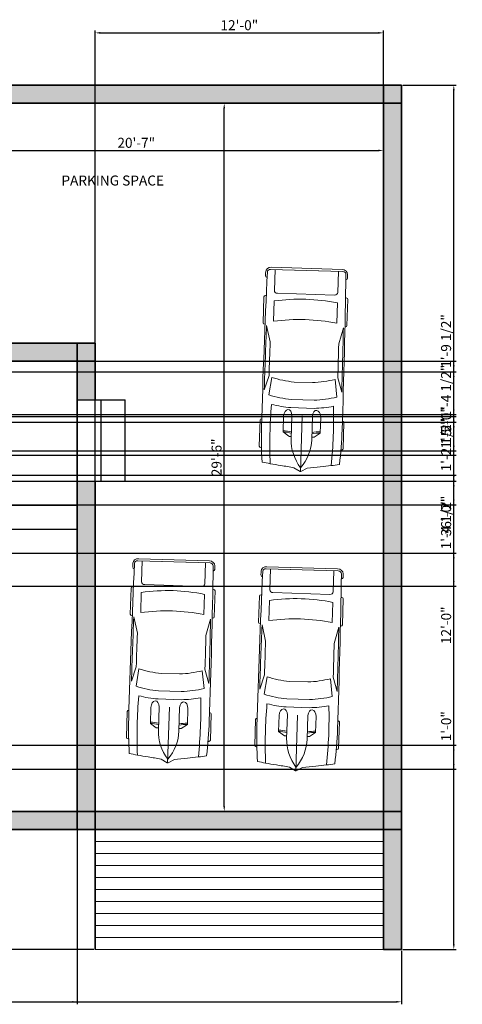
# Model space of a CAD drawing. Units: millimetres. Extents: x 2803 to 3393, y 965 to 1464.
# Tile 6 of 6: x 3172 to 3393, y 968 to 1460. Entities that reach past the tile are written whole.
import ezdxf

# ---------------------------------------------------------------- set-up
doc = ezdxf.new("R2010")
doc.units = ezdxf.units.MM
for name, color, linetype, lineweight in [('A-ANNO-DIMS', 150, 'Continuous', 18), ('A-AREA-IDEN', 200, 'Continuous', 25), ('A-SITE-PVMT', 130, 'Continuous', 18), ('A-SITE-VEHI', 170, 'Continuous', 13), ('A-WALL-PATT', 2, 'Continuous', 13), ('staircase', 130, 'Continuous', 25), ('walls', 2, 'Continuous', 35)]:
    doc.layers.add(name, color=color, linetype=linetype, lineweight=lineweight)
doc.styles.get("Standard").update_dxf_attribs({"font": 'arial.ttf'})
doc.dimstyles.new('ISO-25', dxfattribs={"dimtxt": 5, "dimasz": 2.5, "dimexe": 1.25, "dimexo": 0.625, "dimtad": 1, "dimdec": 0, "dimlunit": 3, "dimtxsty": 'Standard', "dimcen": 2.5, "dimadec": 0, "dimazin": 0, "dimtfac": 1, "dimtdec": 0, "dimtmove": 0, "dimatfit": 3, "dimfxl": 1, "dimarcsym": 0})

# ---------------------------------------------------------------- blocks, each defined once
blk = doc.blocks.new('*U4')
for p, q in [((21.1, 37.41), (21.1, 36.83)), ((46.55, 38.89), (22.35, 38.89)), ((47.8, 37.39), (47.8, 37.41)), ((135.45, 37.07), (135.45, 37.41)), ((136.7, 38.89), (160.9, 38.89)), ((162.15, 37.41), (162.15, 36.77)), ((70.03, 31.54), (86.41, 29.35)), ((87.99, 31.87), (74.76, 35.92)), ((134.31, 35.6), (119.29, 31.78)), ((138.42, 29.35), (157.25, 29.35)), ((186.47, 29.35), (167.01, 29.35)), ((186.47, -33.5), (186.47, 33.5)), ((188.4, -32.76), (188.4, 32.76)), ((164.52, 26.39), (164.52, -26.39)), ((29.77, 9.51), (51.68, 9.51)), ((32.12, 9.51), (32.12, 11.15)), ((32.27, 11.63), (36.13, 17.17)), ((36.13, 17.17), (50.94, 17.17)), ((58.92, -10.77), (58.92, 10.77)), ((66.55, -10.53), (66.55, 10.53)), ((186.47, -10.53), (186.47, 10.53)), ((3.27, 6.13), (0.1, 0.41)), ((82.74, 8.5), (82.74, -8.5)), ((0, 0), (51.68, 0)), ((0.1, -0.41), (3.27, -6.13)), ((29.77, -9.51), (51.68, -9.51)), ((32.12, -9.51), (32.12, -11.15)), ((32.27, -11.63), (36.13, -17.17)), ((36.13, -17.17), (50.94, -17.17)), ((86.41, -29.35), (70.03, -31.54)), ((87.99, -31.87), (74.76, -35.92)), ((134.31, -35.6), (119.29, -31.78)), ((157.25, -29.35), (138.42, -29.35)), ((167.01, -29.35), (186.47, -29.35)), ((21.1, -37.41), (21.1, -36.83)), ((46.55, -38.89), (22.35, -38.89)), ((47.8, -37.39), (47.8, -37.41)), ((135.45, -37.07), (135.45, -37.41)), ((136.7, -38.89), (160.9, -38.89)), ((162.15, -37.41), (162.15, -36.77))]:
    blk.add_line(p, q)
for centre, major_axis, ratio, start_param, end_param in [((41.19, -490.86), (0, 528.23), 0.842304, 0.00281, 0.075598), ((22.35, 37.41), (0, -1.48), 0.842304, 3.141593, 4.712389), ((64.48, -10555.62), (0, 10593.03), 0.842304, -0.013397, 0.002797), ((46.55, 37.41), (0, 1.48), 0.842304, -1.570796, 0), ((136.7, 37.41), (0, -1.48), 0.842304, 3.141593, 4.712389), ((160.9, 37.41), (0, 1.48), 0.842304, -1.570796, 0), ((180.63, 35.84), (0, 2.22), 0.842304, -0.013017, 1.249894), ((64.48, -10556.36), (0, 10595.31), 0.842304, -0.013397, -0.013017), ((183.98, 32.76), (0, -5.25), 0.842304, 1.570796, 3.128196), ((259.18, -27.52), (0, -305.3), 0.842304, 4.528606, 4.561838), ((266.03, -27.52), (0, 313.31), 0.842304, 1.367076, 1.39176), ((37.47, -593.96), (0, -623.33), 0.842304, 3.096046, 3.200911), ((134.4, 5.39), (0, -89.78), 0.842304, 4.449482, 4.652344), ((135.29, 5.39), (0, 81.77), 0.842304, 1.245306, 1.50788), ((64.48, -10555.62), (0, -10591.55), 0.842304, 3.133765, 3.140441), ((149.6, 2.8), (0, -79.58), 0.842304, 4.372215, 4.640744), ((95.79, -3666.35), (0, -3698.24), 0.842304, 3.134049, 3.144098), ((17.08, 0), (0, 147.02), 0.842304, 4.511394, 4.913384), ((35.91, 0), (0, 147.02), 0.842304, 4.511394, 4.913384), ((167.01, 26.39), (0, 2.96), 0.842304, 0, 1.570796), ((183.98, 33.5), (0, -2.96), 0.842304, 1.570796, 3.128196), ((-204.49, 52.4), (0, -250.96), 0.842304, 1.385369, 1.434372), ((29.77, -46.66), (0, 56.17), 0.842304, 0, 0.590319), ((32.75, 11.15), (0, 0.74), 0.842304, 0.879714, 1.570796), ((13.04, 17.01), (0, 27.42), 0.842304, 4.435146, 4.718221), ((14.2, 17.01), (0, 27.42), 0.842304, 4.435146, 4.718221), ((50.79, 13.34), (6.34, -0.36), 0.603834, -1.395552, 1.581315), ((0.62, 0), (0, -0.74), 0.842304, 4.131459, 5.293319), ((-204.49, -52.4), (0, 250.96), 0.842304, -1.434372, -1.385369), ((29.77, 46.66), (0, 56.17), 0.842304, 2.551274, 3.141593), ((149.6, -2.8), (0, -79.58), 0.842304, -1.499151, -1.230623), ((32.75, -11.15), (0, -0.74), 0.842304, 4.712389, 5.403472), ((13.04, -17.01), (0, -27.42), 0.842304, 1.564964, 1.848039), ((14.2, -17.01), (0, -27.42), 0.842304, 1.564964, 1.848039), ((134.4, -5.39), (0, -89.78), 0.842304, -1.510751, -1.307889), ((135.29, -5.39), (0, -81.77), 0.842304, -1.50788, -1.245306), ((259.18, 27.52), (0, 305.3), 0.842304, 1.721348, 1.754579), ((167.01, -26.39), (0, -2.96), 0.842304, 4.712389, 6.283185), ((266.03, 27.52), (0, 313.31), 0.842304, 1.749832, 1.774517), ((37.47, 593.96), (0, -623.33), 0.842304, -0.059319, 0.045547), ((41.19, 490.86), (0, -528.23), 0.842304, -0.075598, -0.00281), ((64.48, 10555.62), (0, 10593.03), 0.842304, 3.138796, 3.15499), ((64.48, 10555.62), (0, -10591.55), 0.842304, 0.001152, 0.007828), ((95.79, 3666.35), (0, -3698.24), 0.842304, -0.002505, 0.007544), ((183.98, -33.5), (0, 2.96), 0.842304, 3.15499, 4.712389), ((183.98, -32.76), (0, -5.25), 0.842304, 0.013397, 1.570796), ((22.35, -37.41), (0, 1.48), 0.842304, 1.570796, 3.141593), ((46.55, -37.41), (0, -1.48), 0.842304, 0, 1.570796), ((136.7, -37.41), (0, -1.48), 0.842304, -1.570796, 0), ((160.9, -37.41), (0, 1.48), 0.842304, 3.141593, 4.712389), ((180.63, -35.84), (0, -2.22), 0.842304, -1.249894, 0.013017), ((64.48, 10556.36), (0, 10595.31), 0.842304, 3.15461, 3.15499)]:
    blk.add_ellipse(centre, major_axis=major_axis, ratio=ratio, start_param=start_param, end_param=end_param)
at = {"extrusion": (0, 0, -1)}
blk.add_ellipse((50.79, -13.34), major_axis=(6.34, 0.36), ratio=0.603834, start_param=-1.395552, end_param=1.581315, dxfattribs=at)
blk = doc.blocks.new('*D17')
at = {"layer": 'A-ANNO-DIMS', "color": 0, "lineweight": -2, "transparency": 16777216}
for p, q in [((3106.68, 1401.99), (3106.68, 1393.69)), ((3353.68, 1401.99), (3353.68, 1393.69)), ((3109.18, 1394.94), (3351.18, 1394.94))]:
    blk.add_line(p, q, dxfattribs=at)
at = {"layer": 'A-ANNO-DIMS', "color": 0, "transparency": 16777216}
for points in [[(3109.18, 1395.36), (3109.18, 1394.53), (3106.68, 1394.94)], [(3351.18, 1395.36), (3351.18, 1394.53), (3353.68, 1394.94)]]:
    blk.add_solid(points, dxfattribs=at)
at = {"layer": 'Defpoints', "color": 0, "transparency": 16777216}
for p in [(3106.68, 1402.61), (3353.68, 1402.61), (3353.68, 1394.94)]:
    blk.add_point(p, dxfattribs=at)
at = {"layer": 'A-ANNO-DIMS', "color": 0, "transparency": 16777216, "insert": (3230.18, 1398.12), "char_height": 5, "attachment_point": 5}
blk.add_mtext('20\'-7"', dxfattribs=at)
blk = doc.blocks.new('*D18')
at = {"layer": 'A-ANNO-DIMS', "color": 0, "lineweight": -2, "transparency": 16777216}
for p, q in [((3274.76, 1418.56), (3275.39, 1418.56)), ((3274.14, 1067.06), (3274.14, 1416.06)), ((3278.22, 1064.56), (3272.89, 1064.56))]:
    blk.add_line(p, q, dxfattribs=at)
at = {"layer": 'A-ANNO-DIMS', "color": 0, "transparency": 16777216}
for points in [[(3273.72, 1416.06), (3274.55, 1416.06), (3274.14, 1418.56)], [(3273.72, 1067.06), (3274.55, 1067.06), (3274.14, 1064.56)]]:
    blk.add_solid(points, dxfattribs=at)
at = {"layer": 'Defpoints', "color": 0, "transparency": 16777216}
for p in [(3274.14, 1418.56), (3274.14, 1418.56), (3278.84, 1064.56)]:
    blk.add_point(p, dxfattribs=at)
at = {"layer": 'A-ANNO-DIMS', "color": 0, "transparency": 16777216, "insert": (3270.96, 1241.56), "char_height": 5, "attachment_point": 5, "rotation": 90}
blk.add_mtext('29\'-6"', dxfattribs=at)
blk = doc.blocks.new('*D39')
at = {"layer": 'A-ANNO-DIMS', "color": 0, "lineweight": -2, "transparency": 16777216}
for p, q in [((2839.68, 1023.94), (2839.68, 968.15)), ((3362.68, 994.94), (3362.68, 968.15)), ((2842.18, 969.4), (3360.18, 969.4))]:
    blk.add_line(p, q, dxfattribs=at)
at = {"layer": 'A-ANNO-DIMS', "color": 0, "transparency": 16777216}
for points in [[(2842.18, 969.82), (2842.18, 968.99), (2839.68, 969.4)], [(3360.18, 969.82), (3360.18, 968.99), (3362.68, 969.4)]]:
    blk.add_solid(points, dxfattribs=at)
at = {"layer": 'Defpoints', "color": 0, "transparency": 16777216}
for p in [(2839.68, 1024.56), (3362.68, 995.56), (3362.68, 969.4)]:
    blk.add_point(p, dxfattribs=at)
at = {"layer": 'A-ANNO-DIMS', "color": 0, "transparency": 16777216, "insert": (3101.18, 972.58), "char_height": 5, "attachment_point": 5}
blk.add_mtext('43\'-7"', dxfattribs=at)
blk = doc.blocks.new('*D40')
at = {"layer": 'A-ANNO-DIMS', "color": 0, "lineweight": -2, "transparency": 16777216}
for p, q in [((3363.31, 1427.56), (3390.09, 1427.56)), ((3388.84, 998.06), (3388.84, 1425.06)), ((3363.31, 995.56), (3390.09, 995.56))]:
    blk.add_line(p, q, dxfattribs=at)
at = {"layer": 'A-ANNO-DIMS', "color": 0, "transparency": 16777216}
for points in [[(3388.43, 1425.06), (3389.26, 1425.06), (3388.84, 1427.56)], [(3388.43, 998.06), (3389.26, 998.06), (3388.84, 995.56)]]:
    blk.add_solid(points, dxfattribs=at)
at = {"layer": 'Defpoints', "color": 0, "transparency": 16777216}
for p in [(3362.68, 1427.56), (3388.84, 1427.56), (3362.68, 995.56)]:
    blk.add_point(p, dxfattribs=at)
at = {"layer": 'A-ANNO-DIMS', "color": 0, "transparency": 16777216, "insert": (3385.66, 1211.56), "char_height": 5, "attachment_point": 5, "rotation": 90}
blk.add_mtext('36\'-0"', dxfattribs=at)
blk = doc.blocks.new('*D41')
at = {"layer": 'A-ANNO-DIMS', "color": 0, "lineweight": -2, "transparency": 16777216}
for p, q in [((3209.68, 1056.19), (3209.68, 1454.97)), ((3212.18, 1453.72), (3351.18, 1453.72)), ((3353.68, 1056.19), (3353.68, 1454.97))]:
    blk.add_line(p, q, dxfattribs=at)
at = {"layer": 'A-ANNO-DIMS', "color": 0, "transparency": 16777216}
for points in [[(3212.18, 1454.14), (3212.18, 1453.31), (3209.68, 1453.72)], [(3351.18, 1454.14), (3351.18, 1453.31), (3353.68, 1453.72)]]:
    blk.add_solid(points, dxfattribs=at)
at = {"layer": 'Defpoints', "color": 0, "transparency": 16777216}
for p in [(3353.68, 1453.72), (3209.68, 1055.56), (3353.68, 1055.56)]:
    blk.add_point(p, dxfattribs=at)
at = {"layer": 'A-ANNO-DIMS', "color": 0, "transparency": 16777216, "insert": (3281.68, 1456.9), "char_height": 5, "attachment_point": 5}
blk.add_mtext('12\'-0"', dxfattribs=at)
blk = doc.blocks.new('*D42')
at = {"layer": 'A-ANNO-DIMS', "color": 0, "lineweight": -2, "transparency": 16777216}
for p, q in [((3209.06, 1055.56), (2812.27, 1055.56)), ((2813.52, 998.06), (2813.52, 1053.06)), ((3209.06, 995.56), (2812.27, 995.56))]:
    blk.add_line(p, q, dxfattribs=at)
at = {"layer": 'A-ANNO-DIMS', "color": 0, "transparency": 16777216}
for points in [[(2813.11, 1053.06), (2813.94, 1053.06), (2813.52, 1055.56)], [(2813.11, 998.06), (2813.94, 998.06), (2813.52, 995.56)]]:
    blk.add_solid(points, dxfattribs=at)
at = {"layer": 'Defpoints', "color": 0, "transparency": 16777216}
for p in [(2813.52, 1055.56), (3209.68, 1055.56), (3209.68, 995.56)]:
    blk.add_point(p, dxfattribs=at)
at = {"layer": 'A-ANNO-DIMS', "color": 0, "transparency": 16777216, "insert": (2810.35, 1025.56), "char_height": 5, "attachment_point": 5, "rotation": 90}
blk.add_mtext('5\'-0"', dxfattribs=at)
blk = doc.blocks.new('*D44')
at = {"layer": 'A-ANNO-DIMS', "color": 0, "lineweight": -2, "transparency": 16777216}
for p, q in [((3148.87, 1229.61), (3390.09, 1229.61)), ((3388.84, 1088.11), (3388.84, 1227.11)), ((3148.87, 1085.61), (3390.09, 1085.61))]:
    blk.add_line(p, q, dxfattribs=at)
at = {"layer": 'A-ANNO-DIMS', "color": 0, "transparency": 16777216}
for points in [[(3388.43, 1227.11), (3389.26, 1227.11), (3388.84, 1229.61)], [(3388.43, 1088.11), (3389.26, 1088.11), (3388.84, 1085.61)]]:
    blk.add_solid(points, dxfattribs=at)
at = {"layer": 'Defpoints', "color": 0, "transparency": 16777216}
for p in [(3148.25, 1229.61), (3388.84, 1229.61), (3148.25, 1085.61)]:
    blk.add_point(p, dxfattribs=at)
at = {"layer": 'A-ANNO-DIMS', "color": 0, "transparency": 16777216, "insert": (3385.67, 1157.61), "char_height": 5, "attachment_point": 5, "rotation": 90}
blk.add_mtext('12\'-0"', dxfattribs=at)
blk = doc.blocks.new('*D45')
at = {"layer": 'A-ANNO-DIMS', "color": 0, "lineweight": -2, "transparency": 16777216}
for p, q in [((3200.68, 1297.94), (3200.68, 968.15)), ((3106.68, 1288.94), (3106.68, 968.15)), ((3109.18, 969.4), (3198.18, 969.4))]:
    blk.add_line(p, q, dxfattribs=at)
at = {"layer": 'A-ANNO-DIMS', "color": 0, "transparency": 16777216}
for points in [[(3109.18, 969.82), (3109.18, 968.99), (3106.68, 969.4)], [(3198.18, 969.82), (3198.18, 968.99), (3200.68, 969.4)]]:
    blk.add_solid(points, dxfattribs=at)
at = {"layer": 'Defpoints', "color": 0, "transparency": 16777216}
for p in [(3200.68, 1298.56), (3106.68, 1289.56), (3200.68, 969.4)]:
    blk.add_point(p, dxfattribs=at)
at = {"layer": 'A-ANNO-DIMS', "color": 0, "transparency": 16777216, "insert": (3153.68, 972.58), "char_height": 5, "attachment_point": 5}
blk.add_mtext('7\'-10"', dxfattribs=at)
blk = doc.blocks.new('*D46')
at = {"layer": 'A-ANNO-DIMS', "color": 0, "lineweight": -2, "transparency": 16777216}
for p, q in [((3067.93, 1289.56), (3390.09, 1289.56)), ((3388.84, 1232.11), (3388.84, 1287.06)), ((3201.31, 1229.61), (3390.09, 1229.61))]:
    blk.add_line(p, q, dxfattribs=at)
at = {"layer": 'A-ANNO-DIMS', "color": 0, "transparency": 16777216}
for points in [[(3388.43, 1287.06), (3389.26, 1287.06), (3388.84, 1289.56)], [(3388.43, 1232.11), (3389.26, 1232.11), (3388.84, 1229.61)]]:
    blk.add_solid(points, dxfattribs=at)
at = {"layer": 'Defpoints', "color": 0, "transparency": 16777216}
for p in [(3067.31, 1289.56), (3388.84, 1289.56), (3200.68, 1229.61)]:
    blk.add_point(p, dxfattribs=at)
at = {"layer": 'A-ANNO-DIMS', "color": 0, "transparency": 16777216, "insert": (3385.67, 1259.59), "char_height": 5, "attachment_point": 5, "rotation": 90}
blk.add_mtext('5\'-0"', dxfattribs=at)
blk = doc.blocks.new('*D47')
at = {"layer": 'A-ANNO-DIMS', "color": 0, "lineweight": -2, "transparency": 16777216}
for p, q in [((3388.84, 1097.61), (3388.84, 1114.18)), ((3143.31, 1097.61), (3390.09, 1097.61)), ((3388.84, 1088.11), (3388.84, 1095.11)), ((3143.31, 1085.61), (3390.09, 1085.61))]:
    blk.add_line(p, q, dxfattribs=at)
at = {"layer": 'A-ANNO-DIMS', "color": 0, "transparency": 16777216}
for points in [[(3388.43, 1095.11), (3389.26, 1095.11), (3388.84, 1097.61)], [(3388.43, 1088.11), (3389.26, 1088.11), (3388.84, 1085.61)]]:
    blk.add_solid(points, dxfattribs=at)
at = {"layer": 'Defpoints', "color": 0, "transparency": 16777216}
for p in [(3142.68, 1097.61), (3388.84, 1097.61), (3142.68, 1085.61)]:
    blk.add_point(p, dxfattribs=at)
at = {"layer": 'A-ANNO-DIMS', "color": 0, "transparency": 16777216, "insert": (3385.67, 1107.15), "char_height": 5, "attachment_point": 5, "rotation": 90}
blk.add_mtext('1\'-0"', dxfattribs=at)
blk = doc.blocks.new('*D66')
at = {"layer": 'A-ANNO-DIMS', "color": 0, "lineweight": -2, "transparency": 16777216}
for p, q in [((3022.85, 1262), (3390.09, 1262)), ((3388.84, 1247.31), (3388.84, 1259.5)), ((3022.85, 1244.81), (3390.09, 1244.81))]:
    blk.add_line(p, q, dxfattribs=at)
at = {"layer": 'A-ANNO-DIMS', "color": 0, "transparency": 16777216}
for points in [[(3388.43, 1259.5), (3389.26, 1259.5), (3388.84, 1262)], [(3388.43, 1247.31), (3389.26, 1247.31), (3388.84, 1244.81)]]:
    blk.add_solid(points, dxfattribs=at)
at = {"layer": 'Defpoints', "color": 0, "transparency": 16777216}
for p in [(3022.23, 1262), (3388.84, 1262), (3022.23, 1244.81)]:
    blk.add_point(p, dxfattribs=at)
at = {"layer": 'A-ANNO-DIMS', "color": 0, "transparency": 16777216, "insert": (3385.67, 1253.41), "char_height": 5, "attachment_point": 5, "rotation": 90}
blk.add_mtext('1\'-5"', dxfattribs=at)
blk = doc.blocks.new('*D68')
at = {"layer": 'A-ANNO-DIMS', "color": 0, "lineweight": -2, "transparency": 16777216}
for p, q in [((3388.84, 1259.07), (3388.84, 1287.29)), ((2942.31, 1259.07), (3390.09, 1259.07)), ((3388.84, 1245.09), (3388.84, 1256.57)), ((2942.31, 1242.59), (3390.09, 1242.59))]:
    blk.add_line(p, q, dxfattribs=at)
at = {"layer": 'A-ANNO-DIMS', "color": 0, "transparency": 16777216}
for points in [[(3388.43, 1256.57), (3389.26, 1256.57), (3388.84, 1259.07)], [(3388.43, 1245.09), (3389.26, 1245.09), (3388.84, 1242.59)]]:
    blk.add_solid(points, dxfattribs=at)
at = {"layer": 'Defpoints', "color": 0, "transparency": 16777216}
for p in [(2941.68, 1259.07), (3388.84, 1259.07), (2941.68, 1242.59)]:
    blk.add_point(p, dxfattribs=at)
at = {"layer": 'A-ANNO-DIMS', "color": 0, "transparency": 16777216, "insert": (3385.63, 1274.43), "char_height": 5, "attachment_point": 5, "rotation": 90}
blk.add_mtext('1\'-4 1/2"', dxfattribs=at)
blk = doc.blocks.new('*D69')
at = {"layer": 'A-ANNO-DIMS', "color": 0, "lineweight": -2, "transparency": 16777216}
for p, q in [((3388.84, 1193.62), (3388.84, 1221.84)), ((2942.31, 1193.62), (3390.09, 1193.62)), ((3388.84, 1179.64), (3388.84, 1191.12)), ((2942.31, 1177.14), (3390.09, 1177.14))]:
    blk.add_line(p, q, dxfattribs=at)
at = {"layer": 'A-ANNO-DIMS', "color": 0, "transparency": 16777216}
for points in [[(3388.43, 1191.12), (3389.26, 1191.12), (3388.84, 1193.62)], [(3388.43, 1179.64), (3389.26, 1179.64), (3388.84, 1177.14)]]:
    blk.add_solid(points, dxfattribs=at)
at = {"layer": 'Defpoints', "color": 0, "transparency": 16777216}
for p in [(2941.68, 1193.62), (3388.84, 1193.62), (2941.68, 1177.14)]:
    blk.add_point(p, dxfattribs=at)
at = {"layer": 'A-ANNO-DIMS', "color": 0, "transparency": 16777216, "insert": (3385.63, 1208.98), "char_height": 5, "attachment_point": 5, "rotation": 90}
blk.add_mtext('1\'-4 1/2"', dxfattribs=at)
blk = doc.blocks.new('*D72')
at = {"layer": 'A-ANNO-DIMS', "color": 0, "lineweight": -2, "transparency": 16777216}
for p, q in [((3388.84, 1284.35), (3388.84, 1312.57)), ((3107.31, 1284.35), (3390.09, 1284.35)), ((3388.84, 1265.46), (3388.84, 1281.85)), ((3107.31, 1262.96), (3390.09, 1262.96))]:
    blk.add_line(p, q, dxfattribs=at)
at = {"layer": 'A-ANNO-DIMS', "color": 0, "transparency": 16777216}
for points in [[(3388.43, 1281.85), (3389.26, 1281.85), (3388.84, 1284.35)], [(3388.43, 1265.46), (3389.26, 1265.46), (3388.84, 1262.96)]]:
    blk.add_solid(points, dxfattribs=at)
at = {"layer": 'Defpoints', "color": 0, "transparency": 16777216}
for p in [(3106.68, 1284.35), (3388.84, 1284.35), (3106.68, 1262.96)]:
    blk.add_point(p, dxfattribs=at)
at = {"layer": 'A-ANNO-DIMS', "color": 0, "transparency": 16777216, "insert": (3385.63, 1299.71), "char_height": 5, "attachment_point": 5, "rotation": 90}
blk.add_mtext('1\'-9 1/2"', dxfattribs=at)
blk = doc.blocks.new('*D74')
at = {"layer": 'A-ANNO-DIMS', "color": 0, "lineweight": -2, "transparency": 16777216}
for p, q in [((3388.84, 1232.56), (3388.84, 1260.78)), ((2869.11, 1232.56), (3390.09, 1232.56)), ((3388.84, 1220.39), (3388.84, 1230.06)), ((2933.31, 1217.89), (3390.09, 1217.89))]:
    blk.add_line(p, q, dxfattribs=at)
at = {"layer": 'A-ANNO-DIMS', "color": 0, "transparency": 16777216}
for points in [[(3388.43, 1230.06), (3389.26, 1230.06), (3388.84, 1232.56)], [(3388.43, 1220.39), (3389.26, 1220.39), (3388.84, 1217.89)]]:
    blk.add_solid(points, dxfattribs=at)
at = {"layer": 'Defpoints', "color": 0, "transparency": 16777216}
for p in [(2868.49, 1232.56), (3388.84, 1232.56), (2932.68, 1217.89)]:
    blk.add_point(p, dxfattribs=at)
at = {"layer": 'A-ANNO-DIMS', "color": 0, "transparency": 16777216, "insert": (3385.63, 1247.92), "char_height": 5, "attachment_point": 5, "rotation": 90}
blk.add_mtext('1\'-2 1/2"', dxfattribs=at)

msp = doc.modelspace()

# ---------------------------------------------------------------- hatches: boundary and pattern name
at = {"layer": 'A-WALL-PATT'}
h = msp.add_hatch(color=256, dxfattribs=at)
h.dxf.hatch_style = 1
h.paths.add_polyline_path([(2968.68, 1427.56), (2919.98, 1427.56), (2919.98, 1418.56), (2968.68, 1418.56)])
h.paths.add_polyline_path([(2977.68, 1427.56), (2968.68, 1427.56), (2968.68, 1418.56), (2977.68, 1418.56)])
h.paths.add_polyline_path([(2977.68, 1418.56), (2968.68, 1418.56), (2968.68, 1298.56), (2977.68, 1298.56)])
h.paths.add_polyline_path([(3021.74, 1427.56), (2977.68, 1427.56), (2977.68, 1418.56), (3021.74, 1418.56)])
h.paths.add_polyline_path([(2881.7, 1427.56), (2848.68, 1427.56), (2848.68, 1418.56), (2881.7, 1418.56)])
h.paths.add_polyline_path([(2848.68, 1427.56), (2839.68, 1427.56), (2839.68, 1418.56), (2848.68, 1418.56)])
h.paths.add_polyline_path([(2848.68, 1418.56), (2839.68, 1418.56), (2839.68, 1298.56), (2848.68, 1298.56)])
h.paths.add_polyline_path([(2932.68, 1298.56), (2848.68, 1298.56), (2848.68, 1289.56), (2932.68, 1289.56)])
h.paths.add_polyline_path([(2848.68, 1298.56), (2839.68, 1298.56), (2839.68, 1289.56), (2848.68, 1289.56)])
h.paths.add_polyline_path([(2848.68, 1289.56), (2839.68, 1289.56), (2839.68, 1280.88), (2848.68, 1280.88)])
h.paths.add_polyline_path([(2848.68, 1252.94), (2839.68, 1252.94), (2839.68, 1241.56), (2848.68, 1241.56)])
h.paths.add_polyline_path([(2848.68, 1241.56), (2839.68, 1241.56), (2839.68, 1232.56), (2848.68, 1232.56)])
h.paths.add_polyline_path([(2932.68, 1241.56), (2848.68, 1241.56), (2848.68, 1232.56), (2932.68, 1232.56)])
h.paths.add_polyline_path([(2941.68, 1241.56), (2932.68, 1241.56), (2932.68, 1232.56), (2941.68, 1232.56)])
h.paths.add_polyline_path([(2941.68, 1289.56), (2932.68, 1289.56), (2932.68, 1257.22, -0.114666), (2939.92, 1259.03), (2941.68, 1259.07)])
h.paths.add_polyline_path([(2941.68, 1298.56), (2932.68, 1298.56), (2932.68, 1289.56), (2941.68, 1289.56)])
h.paths.add_polyline_path([(2947.42, 1298.56), (2941.68, 1298.56), (2941.68, 1289.56), (2945.75, 1289.56), (2945.75, 1290.29, -0.099582)])
h.paths.add_polyline_path([(2977.68, 1298.56), (2968.68, 1298.56), (2968.68, 1289.56), (2977.68, 1289.56)])
h.paths.add_polyline_path([(3018.47, 1298.56), (2977.68, 1298.56), (2977.68, 1289.56), (3018.47, 1289.56)])
h.paths.add_polyline_path([(3097.68, 1298.56), (3067.31, 1298.56), (3067.31, 1289.56), (3097.68, 1289.56)])
h.paths.add_polyline_path([(3106.68, 1298.56), (3097.68, 1298.56), (3097.68, 1289.56), (3106.68, 1289.56)])
h.paths.add_polyline_path([(3200.68, 1298.56), (3106.68, 1298.56), (3106.68, 1289.56), (3200.68, 1289.56)])
h.paths.add_polyline_path([(3209.68, 1298.56), (3200.68, 1298.56), (3200.68, 1289.56), (3209.68, 1289.56)])
h.paths.add_polyline_path([(3209.68, 1289.56), (3200.68, 1289.56), (3200.68, 1270.22), (3209.68, 1270.22)])
h.paths.add_polyline_path([(3106.68, 1418.56), (3097.68, 1418.56), (3097.68, 1298.56), (3106.68, 1298.56)])
h.paths.add_polyline_path([(3106.68, 1427.56), (3097.68, 1427.56), (3097.68, 1418.56), (3106.68, 1418.56)])
h.paths.add_polyline_path([(3097.68, 1427.56), (3058.94, 1427.56), (3058.94, 1418.56), (3097.68, 1418.56)])
h.paths.add_polyline_path([(3353.68, 1427.56), (3106.68, 1427.56), (3106.68, 1418.56), (3353.68, 1418.56)])
h.paths.add_polyline_path([(3362.68, 1427.56), (3353.68, 1427.56), (3353.68, 1418.56), (3362.68, 1418.56)])
h.paths.add_polyline_path([(3362.68, 1418.56), (3353.68, 1418.56), (3353.68, 1064.56), (3362.68, 1064.56)])
h.paths.add_polyline_path([(3362.68, 1064.56), (3353.68, 1064.56), (3353.68, 1055.56), (3362.68, 1055.56)])
h.paths.add_polyline_path([(3362.68, 1055.56), (3353.68, 1055.56), (3353.68, 995.56), (3362.68, 995.56)])
h.paths.add_polyline_path([(3353.68, 1064.56), (3209.68, 1064.56), (3209.68, 1055.56), (3353.68, 1055.56)])
h.paths.add_polyline_path([(3200.68, 1064.56), (3106.68, 1064.56), (3106.68, 1055.56), (3200.68, 1055.56)])
h.paths.add_polyline_path([(3209.68, 1064.56), (3200.68, 1064.56), (3200.68, 1055.56), (3209.68, 1055.56)])
h.paths.add_polyline_path([(3209.68, 1229.61), (3200.68, 1229.61), (3200.68, 1064.56), (3209.68, 1064.56)])
h.paths.add_polyline_path([(3106.68, 1117.56), (3097.68, 1117.56), (3097.68, 1064.56), (3106.68, 1064.56)])
h.paths.add_polyline_path([(3106.68, 1126.56), (3097.68, 1126.56), (3097.68, 1117.56), (3106.68, 1117.56)])
h.paths.add_polyline_path([(3097.68, 1126.56), (3001.68, 1126.56), (3001.68, 1117.56), (3097.68, 1117.56)])
h.paths.add_polyline_path([(3001.68, 1165.56), (2992.68, 1165.56), (2992.68, 1126.56), (3001.68, 1126.56)])
h.paths.add_polyline_path([(3001.68, 1174.56), (2992.68, 1174.56), (2992.68, 1165.56), (3001.68, 1165.56)])
h.paths.add_polyline_path([(2992.68, 1174.56), (2986.69, 1174.56), (2986.69, 1165.56), (2992.68, 1165.56)])
h.paths.add_polyline_path([(3001.68, 1126.56), (2992.68, 1126.56), (2992.68, 1117.56), (3001.68, 1117.56)])
h.paths.add_polyline_path([(3001.68, 1117.56), (2992.68, 1117.56), (2992.68, 1112.21), (2994.15, 1112.23), (3001.68, 1112.37)])
h.paths.add_polyline_path([(3001.68, 1033.56), (2992.68, 1033.56), (2992.68, 1024.56), (3001.68, 1024.56)])
h.paths.add_polyline_path([(3001.68, 1097.58, -0.114732), (2994.45, 1095.76), (2992.68, 1095.73), (2992.68, 1033.56), (3001.68, 1033.56)])
h.paths.add_polyline_path([(3030.4, 1033.56), (3001.68, 1033.56), (3001.68, 1024.56), (3030.4, 1024.56)])
h.paths.add_polyline_path([(3097.68, 1033.56), (3060.2, 1033.56), (3060.2, 1024.56), (3097.68, 1024.56)])
h.paths.add_polyline_path([(3106.68, 1033.56), (3097.68, 1033.56), (3097.68, 1024.56), (3106.68, 1024.56)])
h.paths.add_polyline_path([(3106.68, 1055.56), (3097.68, 1055.56), (3097.68, 1033.56), (3106.68, 1033.56)])
h.paths.add_polyline_path([(3106.68, 1064.56), (3097.68, 1064.56), (3097.68, 1055.56), (3106.68, 1055.56)])
h.paths.add_polyline_path([(2992.68, 1033.56), (2848.68, 1033.56), (2848.68, 1024.56), (2992.68, 1024.56)])
h.paths.add_polyline_path([(2848.68, 1033.56), (2839.68, 1033.56), (2839.68, 1024.56), (2848.68, 1024.56)])
h.paths.add_polyline_path([(2848.68, 1070.54), (2839.68, 1070.54), (2839.68, 1033.56), (2848.68, 1033.56)])
h.paths.add_polyline_path([(2848.68, 1165.56), (2839.68, 1165.56), (2839.68, 1114.52), (2848.68, 1114.52)])
h.paths.add_polyline_path([(2848.68, 1174.56), (2839.68, 1174.56), (2839.68, 1165.56), (2848.68, 1165.56)])
h.paths.add_polyline_path([(2932.68, 1174.56), (2848.68, 1174.56), (2848.68, 1165.56), (2932.68, 1165.56)])
h.paths.add_polyline_path([(2941.68, 1174.56), (2932.68, 1174.56), (2932.68, 1165.56), (2941.68, 1165.56)])
h.paths.add_polyline_path([(2965.38, 1174.56), (2941.68, 1174.56), (2941.68, 1165.56), (2968.2, 1165.56, -0.111634)])
h.paths.add_polyline_path([(2848.68, 1193.13), (2839.68, 1193.13), (2839.68, 1174.56), (2848.68, 1174.56)])
h.paths.add_polyline_path([(2848.68, 1232.56), (2839.68, 1232.56), (2839.68, 1221.86), (2848.68, 1221.86)])
h.paths.add_polyline_path([(2941.68, 1232.56), (2932.68, 1232.56), (2932.68, 1191.24, -0.132111), (2940.91, 1193.6), (2941.68, 1193.62)])
h.paths.add_polyline_path([(3106.68, 1262.96), (3105.94, 1262.96, -0.099353), (3097.68, 1264.61), (3097.68, 1126.56), (3106.68, 1126.56)])

# ---------------------------------------------------------------- linework, layer by layer
at = {"layer": 'A-SITE-PVMT'}
for p, q in [((3209.68, 1055.56), (3353.68, 1055.56)), ((3209.68, 1049.56), (3353.68, 1049.56)), ((3209.68, 1043.56), (3353.68, 1043.56)), ((3209.68, 1037.56), (3353.68, 1037.56)), ((3209.68, 1031.56), (3353.68, 1031.56)), ((3209.68, 1025.56), (3353.68, 1025.56)), ((3209.68, 1019.56), (3353.68, 1019.56)), ((3209.68, 1013.56), (3353.68, 1013.56)), ((3209.68, 1007.56), (3353.68, 1007.56)), ((3209.68, 1001.56), (3353.68, 1001.56)), ((3209.68, 995.56), (3353.68, 995.56))]:
    msp.add_line(p, q, dxfattribs=at)
at = {"layer": 'staircase'}
for p, q in [((3200.68, 1229.61), (3200.68, 1270.22)), ((3200.68, 1270.22), (3224.68, 1270.22)), ((3212.68, 1229.61), (3212.68, 1270.22)), ((3224.68, 1229.61), (3224.68, 1270.22)), ((3106.68, 1229.61), (3200.68, 1229.61)), ((3200.68, 1229.61), (3224.68, 1229.61)), ((3106.68, 1217.61), (3200.68, 1217.61)), ((3106.68, 1205.61), (3200.68, 1205.61)), ((3106.68, 1193.61), (3200.68, 1193.61))]:
    msp.add_line(p, q, dxfattribs=at)
at = {"layer": 'walls'}
for p, q in [((2839.68, 1427.56), (3362.68, 1427.56)), ((3353.68, 1427.56), (3353.68, 995.56)), ((3362.68, 1427.56), (3362.68, 995.56)), ((2839.68, 1418.56), (3362.68, 1418.56)), ((3106.68, 1298.56), (3209.68, 1298.56)), ((3200.68, 1298.56), (3200.68, 1055.56)), ((3209.68, 1298.56), (3209.68, 1270.22)), ((3106.68, 1289.56), (3209.68, 1289.56)), ((3209.68, 1229.61), (3209.68, 995.56)), ((3097.68, 1064.56), (3362.68, 1064.56)), ((3097.68, 1055.56), (3362.68, 1055.56)), ((3353.68, 995.56), (3362.68, 995.56))]:
    msp.add_line(p, q, dxfattribs=at)

# ---------------------------------------------------------------- block references
at = {"layer": 'A-SITE-VEHI', "xscale": 0.5390619056293562, "yscale": 0.5390619056293562, "zscale": 0.5390619056293562, "rotation": 88.20683608042523}
for p in [(3312.22, 1234.48), (3245.87, 1088.84), (3309.94, 1084.84)]:
    msp.add_blockref('*U4', p, dxfattribs=at)

# ---------------------------------------------------------------- texts
at = {"layer": 'A-AREA-IDEN', "insert": (3192.79, 1382.42), "char_height": 5, "attachment_point": 1}
msp.add_mtext_dynamic_manual_height_columns('PARKING SPACE ', width=153.2458, gutter_width=12.5, heights=[0], dxfattribs=at)

# ---------------------------------------------------------------- dimensions: what is measured, and where the dimension line sits
at = {"layer": 'A-ANNO-DIMS'}
for base, p1, p2, override, picture, middle in [((3353.68, 1453.72), (3209.68, 1055.56), (3353.68, 1055.56), {"dimdec": 1, "dimlfac": 1, "dimrnd": 0, "dimzin": 1, "dimdsep": 46, "dimlunit": 4, "dimfrac": 2}, '*D41', (3281.68, 1456.9)), ((3353.68, 1394.94), (3106.68, 1402.61), (3353.68, 1402.61), {"dimclrd": 0, "dimclre": 0, "dimclrt": 0}, '*D17', (3230.18, 1398.12)), ((3200.68, 969.4), (3106.68, 1289.56), (3200.68, 1298.56), {"dimdec": 1, "dimlfac": 1, "dimrnd": 0, "dimzin": 1, "dimdsep": 46, "dimlunit": 4, "dimfrac": 2}, '*D45', (3153.68, 972.58)), ((3362.68, 969.4), (2839.68, 1024.56), (3362.68, 995.56), {"dimdec": 1, "dimlfac": 1, "dimrnd": 0, "dimzin": 1, "dimdsep": 46, "dimlunit": 4, "dimfrac": 2}, '*D39', (3101.18, 972.58))]:
    dim = msp.add_linear_dim(base=base, p1=p1, p2=p2, dimstyle='ISO-25', override=override, dxfattribs=at)
    dim.commit()
    dim.dimension.update_dxf_attribs({"geometry": picture, "text_midpoint": middle})
for base, p1, p2, override, picture, middle in [((3388.84, 1427.56), (3362.68, 995.56), (3362.68, 1427.56), {"dimdec": 1, "dimlfac": 1, "dimrnd": 0, "dimzin": 1, "dimdsep": 46, "dimlunit": 4, "dimfrac": 2}, '*D40', (3385.66, 1211.56)), ((3274.14, 1418.56), (3278.84, 1064.56), (3274.14, 1418.56), {"dimclrd": 0, "dimclre": 0, "dimclrt": 0}, '*D18', (3270.96, 1241.56)), ((3388.84, 1284.35), (3106.68, 1262.96), (3106.68, 1284.35), {"dimdec": 1, "dimlfac": 1, "dimrnd": 0, "dimzin": 1, "dimdsep": 46, "dimlunit": 4, "dimfrac": 2}, '*D72', (3385.63, 1299.71)), ((3388.8438, 1289.563), (3200.6838, 1229.614), (3067.3091, 1289.563), {"dimdec": 1, "dimlfac": 1, "dimrnd": 0, "dimzin": 1, "dimdsep": 46, "dimlunit": 4, "dimfrac": 2}, '*D46', (3385.6659, 1259.5885)), ((3388.84, 1259.07), (2941.68, 1242.59), (2941.68, 1259.07), {"dimdec": 1, "dimlfac": 1, "dimrnd": 0, "dimzin": 1, "dimdsep": 46, "dimlunit": 4, "dimfrac": 2}, '*D68', (3385.63, 1274.43)), ((3388.84, 1232.56), (2932.68, 1217.89), (2868.49, 1232.56), {"dimdec": 1, "dimlfac": 1, "dimrnd": 0, "dimzin": 1, "dimdsep": 46, "dimlunit": 4, "dimfrac": 2}, '*D74', (3385.63, 1247.92)), ((3388.84, 1262), (3022.23, 1244.81), (3022.23, 1262), {"dimdec": 1, "dimlfac": 1, "dimrnd": 0, "dimzin": 1, "dimdsep": 46, "dimlunit": 4, "dimfrac": 2}, '*D66', (3385.67, 1253.41)), ((3388.84, 1229.61), (3148.25, 1085.61), (3148.25, 1229.61), {"dimdec": 1, "dimlfac": 1, "dimrnd": 0, "dimzin": 1, "dimdsep": 46, "dimlunit": 4, "dimfrac": 2}, '*D44', (3385.67, 1157.61)), ((3388.84, 1193.62), (2941.68, 1177.14), (2941.68, 1193.62), {"dimdec": 1, "dimlfac": 1, "dimrnd": 0, "dimzin": 1, "dimdsep": 46, "dimlunit": 4, "dimfrac": 2}, '*D69', (3385.63, 1208.98)), ((3388.84, 1097.61), (3142.68, 1085.61), (3142.68, 1097.61), {"dimdec": 1, "dimlfac": 1, "dimrnd": 0, "dimzin": 1, "dimdsep": 46, "dimlunit": 4, "dimfrac": 2}, '*D47', (3385.67, 1107.15)), ((2813.52, 1055.56), (3209.68, 995.56), (3209.68, 1055.56), {"dimdec": 1, "dimlfac": 1, "dimrnd": 0, "dimzin": 1, "dimdsep": 46, "dimlunit": 4, "dimfrac": 2}, '*D42', (2810.35, 1025.56))]:
    dim = msp.add_linear_dim(base=base, p1=p1, p2=p2, angle=90, dimstyle='ISO-25', override=override, dxfattribs=at)
    dim.commit()
    dim.dimension.update_dxf_attribs({"geometry": picture, "text_midpoint": middle})

doc.saveas('drawing.dxf')
